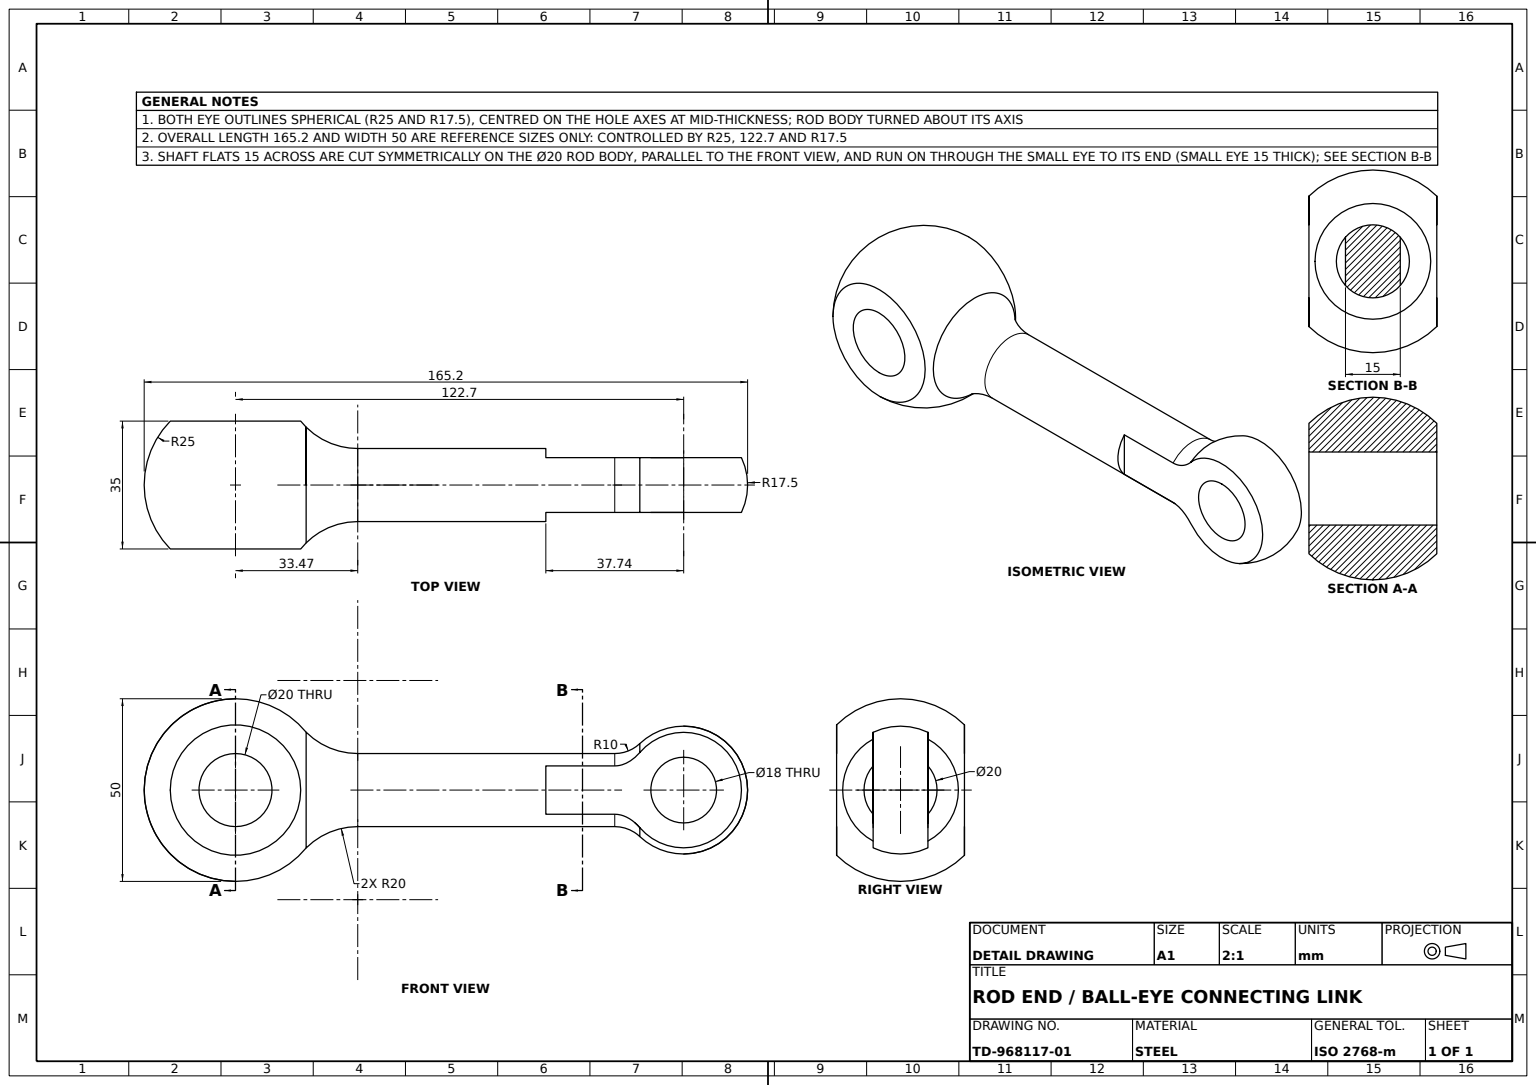
from build123d import *

# Parameters (mm, degrees)
END_BLEND_FILLET_R10_A_R = 10
END_BLEND_FILLET_R10_B_R = 10
SHAFT_FLAT_CUT_REACH     = 101.084
SHAFT_START              = 7.5
SHAFT_FLAT_SKETCH_W      = 28.74
SHAFT_FLAT_SKETCH_H      = 13.228756556


with BuildPart() as part:
    # Rod Revolve Profile → Rod Body Revolve (revolve)
    with BuildSketch(Plane.XY, mode=Mode.PRIVATE) as rod_body_revolve_sk:
        with BuildLine():
            ThreePointArc((-43.496428929, 17.5), (-36.54418797, 11.972243623), (-27.883933933, 10))
            Line((-27.883933933, 10), (52.35, 10))
            Line((52.35, 10), (52.35, 0))
            Line((52.35, 0), (-51.35, 0))
            Line((-51.35, 0), (-51.35, 17.5))
            Line((-51.35, 17.5), (-43.496428929, 17.5))
        make_face()
    revolve(rod_body_revolve_sk.sketch.rotate(Axis((-51.35, 0, 0), (1, 0, 0)), 90), axis=Axis((-51.35, 0, 0), (1, 0, 0)))

    # Sketch5_17 → End Boss Revolve A (revolve)
    with BuildSketch(Plane.XY, mode=Mode.PRIVATE) as end_boss_revolve_a_sk:
        with BuildLine():
            Line((-71.35, 17.5), (-79.203571071, 17.5))
            ThreePointArc((-79.203571071, 17.5), (-86.35, 0), (-79.203571071, -17.5))
            Line((-79.203571071, -17.5), (-71.35, -17.5))
            Line((-71.35, -17.5), (-71.35, 17.5))
        make_face()
    revolve(end_boss_revolve_a_sk.sketch.rotate(Axis((-61.35, -17.5, 0), (0, 1, 0)), 270), axis=Axis((-61.35, -17.5, 0), (0, 1, 0)))

    # Sketch5_18 → End Boss Revolve B (revolve)
    with BuildSketch(Plane.XY, mode=Mode.PRIVATE) as end_boss_revolve_b_sk:
        with BuildLine():
            Line((77.161388301, -7.5), (70.35, -7.5))
            Line((70.35, -7.5), (70.35, 7.5))
            Line((70.35, 7.5), (77.161388301, 7.5))
            ThreePointArc((77.161388301, 7.5), (78.85, 0), (77.161388301, -7.5))
        make_face()
    revolve(end_boss_revolve_b_sk.sketch.rotate(Axis((61.35, 7.5, 0), (0, -1, 0)), 180), axis=Axis((61.35, 7.5, 0), (0, -1, 0)))

    # End Blend Fillet R10 A
    end_blend_fillet_r10_a_edges = [part.edges().sort_by_distance(p)[0] for p in [
        (46.988593384, 4.114378278, 9.114378278),
    ]]
    fillet(end_blend_fillet_r10_a_edges, radius=END_BLEND_FILLET_R10_A_R)

    # End Blend Fillet R10 B
    end_blend_fillet_r10_b_edges = [part.edges().sort_by_distance(p)[0] for p in [
        (46.988593384, 0, -10),
    ]]
    fillet(end_blend_fillet_r10_b_edges, radius=END_BLEND_FILLET_R10_B_R)

    # Shaft Flat Sketch → Shaft Flat Cut (cut, up to next)
    with BuildSketch(Plane(origin=(0, 0, 0), x_dir=(1, 0, 0), z_dir=(0, 1, 0)).offset(SHAFT_START), mode=Mode.PRIVATE) as shaft_flat_cut_sk1:
        with Locations((37.98, 0)):
            Rectangle(SHAFT_FLAT_SKETCH_W, SHAFT_FLAT_SKETCH_H)
    shaft_flat_cut_tool1 = extrude(shaft_flat_cut_sk1.sketch, amount=SHAFT_FLAT_CUT_REACH, mode=Mode.PRIVATE) & part.part
    shaft_flat_cut = shaft_flat_cut_tool1.solids().sort_by_distance((37.98, 7.5, 0))[0]
    add(shaft_flat_cut, mode=Mode.SUBTRACT)

    # Shaft Flat Mirror: Shaft Flat Cut across plane
    add(shaft_flat_cut.mirror(Plane.ZX), mode=Mode.SUBTRACT)


solid = part.part
